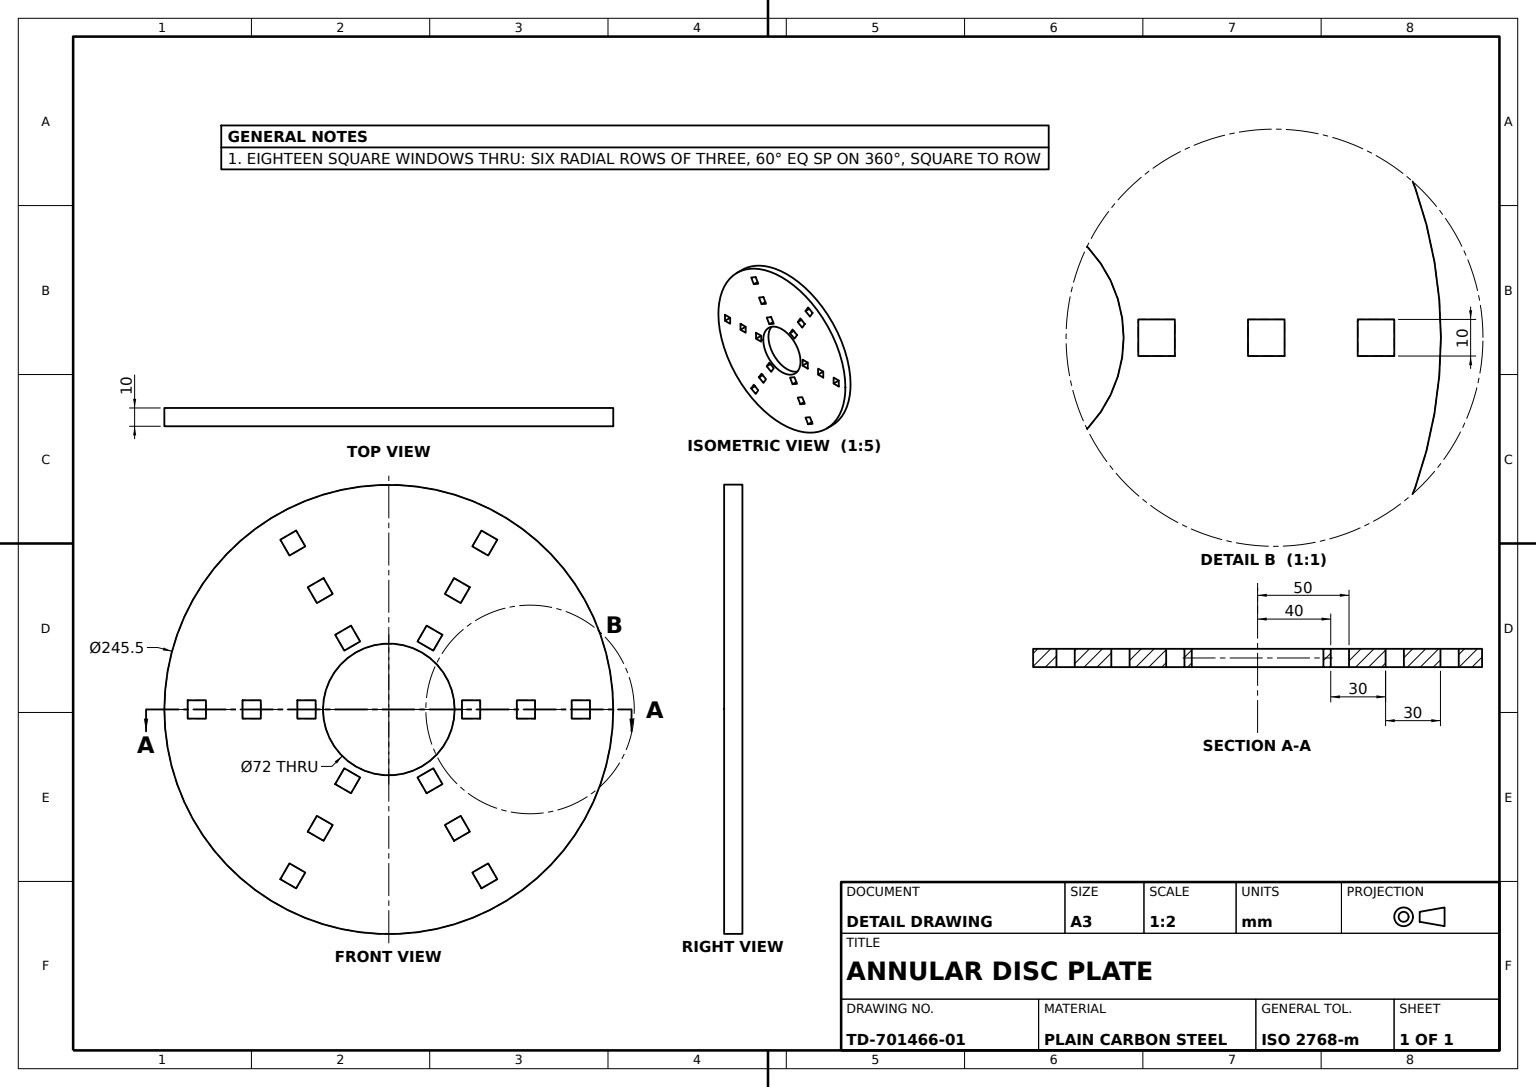
from build123d import *

# Parameters (mm, degrees)
PLATE_PROFILE_245_5_R                        = 122.75
PLATE_DISC_245_5X10_DEPTH                    = 10
CENTRE_BORE_PROFILE_72_R                     = 36
CENTRE_BORE_72_DEPTH                         = 174.882503433
WINDOW_CUT_DEPTH                             = 174.882503433
INNER_WINDOW_CIRCULAR_PATTERN_6X_COUNT       = 6
WINDOW_RADIAL_ROW_3X30_COUNT                 = 3
WINDOW_RADIAL_ROW_3X30_PITCH                 = 30
WINDOW_ROW_CIRCULAR_PATTERN_6X_COPY_1_DEPTH  = 174.882503433
WINDOW_ROW_CIRCULAR_PATTERN_6X_COPY_2_DEPTH  = 174.882503433
WINDOW_ROW_CIRCULAR_PATTERN_6X_COPY_3_DEPTH  = 174.882503433
WINDOW_ROW_CIRCULAR_PATTERN_6X_COPY_4_DEPTH  = 174.882503433
WINDOW_ROW_CIRCULAR_PATTERN_6X_COPY_5_DEPTH  = 174.882503433
WINDOW_ROW_CIRCULAR_PATTERN_6X_COPY_6_DEPTH  = 174.882503433
WINDOW_ROW_CIRCULAR_PATTERN_6X_COPY_7_DEPTH  = 174.882503433
WINDOW_ROW_CIRCULAR_PATTERN_6X_COPY_8_DEPTH  = 174.882503433
WINDOW_ROW_CIRCULAR_PATTERN_6X_COPY_9_DEPTH  = 174.882503433
WINDOW_ROW_CIRCULAR_PATTERN_6X_COPY_10_DEPTH = 174.882503433
WINDOW_ROW_CIRCULAR_PATTERN_6X_COPY_11_DEPTH = 174.882503433
WINDOW_ROW_CIRCULAR_PATTERN_6X_COPY_12_DEPTH = 174.882503433
WINDOW_ROW_CIRCULAR_PATTERN_6X_COPY_13_DEPTH = 174.882503433
WINDOW_ROW_CIRCULAR_PATTERN_6X_COPY_14_DEPTH = 174.882503433
WINDOW_ROW_CIRCULAR_PATTERN_6X_COPY_15_DEPTH = 174.882503433


with BuildPart() as part:
    # Plate Profile Ø245.5 → Plate Disc Ø245.5x10 (new body)
    with BuildSketch(Plane.XY):
        Circle(PLATE_PROFILE_245_5_R)
    extrude(amount=PLATE_DISC_245_5X10_DEPTH)

    # Centre Bore Profile Ø72 → Centre Bore Ø72 (cut, through all)
    with BuildSketch(Plane.XY.offset(10)):
        Circle(CENTRE_BORE_PROFILE_72_R)
    extrude(amount=-CENTRE_BORE_72_DEPTH, mode=Mode.SUBTRACT)

    # Window Profile → Window Cut (cut, through all)
    with BuildSketch(Plane.XY.offset(10)):
        Polygon((50, -5), (50, 5), (40, 5), (40, 0), (40, -5), align=None)
    window_cut = extrude(amount=-WINDOW_CUT_DEPTH, mode=Mode.SUBTRACT)

    # Inner Window Circular Pattern 6x: Window Cut ×6 about axis
    inner_window_circular_pattern_6x_axis = Axis((0, 0, 0), (0, 0, 1))
    for i in range(1, INNER_WINDOW_CIRCULAR_PATTERN_6X_COUNT):
        add(window_cut.rotate(inner_window_circular_pattern_6x_axis, i * 360 / INNER_WINDOW_CIRCULAR_PATTERN_6X_COUNT), mode=Mode.SUBTRACT)

    # Window Radial Row 3x30: Window Cut ×3
    with Locations(*[(i * WINDOW_RADIAL_ROW_3X30_PITCH, 0, 0) for i in range(1, WINDOW_RADIAL_ROW_3X30_COUNT)]):
        add(window_cut, mode=Mode.SUBTRACT)

    # Window Row Circular Pattern 6x copy 1 sk → Window Row Circular Pattern 6x copy 1 (cut, through all)
    with BuildSketch(Plane(origin=(15, 25.980762114, 10), x_dir=(0.5000000000000001, 0.8660254037844386, 0), z_dir=(0, 0, 1))):
        Polygon((50, -5), (50, 5), (40, 5), (40, 0), (40, -5), align=None)
    extrude(amount=-WINDOW_ROW_CIRCULAR_PATTERN_6X_COPY_1_DEPTH, mode=Mode.SUBTRACT)

    # Window Row Circular Pattern 6x copy 2 sk → Window Row Circular Pattern 6x copy 2 (cut, through all)
    with BuildSketch(Plane(origin=(-15, 25.980762114, 10), x_dir=(-0.4999999999999998, 0.8660254037844387, 0), z_dir=(0, 0, 1))):
        Polygon((50, -5), (50, 5), (40, 5), (40, 0), (40, -5), align=None)
    extrude(amount=-WINDOW_ROW_CIRCULAR_PATTERN_6X_COPY_2_DEPTH, mode=Mode.SUBTRACT)

    # Window Row Circular Pattern 6x copy 3 sk → Window Row Circular Pattern 6x copy 3 (cut, through all)
    with BuildSketch(Plane(origin=(-30, 0, 10), x_dir=(-1, 0, 0), z_dir=(0, 0, 1))):
        Polygon((50, -5), (50, 5), (40, 5), (40, 0), (40, -5), align=None)
    extrude(amount=-WINDOW_ROW_CIRCULAR_PATTERN_6X_COPY_3_DEPTH, mode=Mode.SUBTRACT)

    # Window Row Circular Pattern 6x copy 4 sk → Window Row Circular Pattern 6x copy 4 (cut, through all)
    with BuildSketch(Plane(origin=(-15, -25.980762114, 10), x_dir=(-0.5000000000000004, -0.8660254037844384, 0), z_dir=(0, 0, 1))):
        Polygon((50, -5), (50, 5), (40, 5), (40, 0), (40, -5), align=None)
    extrude(amount=-WINDOW_ROW_CIRCULAR_PATTERN_6X_COPY_4_DEPTH, mode=Mode.SUBTRACT)

    # Window Row Circular Pattern 6x copy 5 sk → Window Row Circular Pattern 6x copy 5 (cut, through all)
    with BuildSketch(Plane(origin=(15, -25.980762114, 10), x_dir=(0.5000000000000001, -0.8660254037844386, 0), z_dir=(0, 0, 1))):
        Polygon((50, -5), (50, 5), (40, 5), (40, 0), (40, -5), align=None)
    extrude(amount=-WINDOW_ROW_CIRCULAR_PATTERN_6X_COPY_5_DEPTH, mode=Mode.SUBTRACT)

    # Window Row Circular Pattern 6x copy 6 sk → Window Row Circular Pattern 6x copy 6 (cut, through all)
    with BuildSketch(Plane(origin=(30, 51.961524227, 10), x_dir=(0.5000000000000001, 0.8660254037844386, 0), z_dir=(0, 0, 1))):
        Polygon((50, -5), (50, 5), (40, 5), (40, 0), (40, -5), align=None)
    extrude(amount=-WINDOW_ROW_CIRCULAR_PATTERN_6X_COPY_6_DEPTH, mode=Mode.SUBTRACT)

    # Window Row Circular Pattern 6x copy 7 sk → Window Row Circular Pattern 6x copy 7 (cut, through all)
    with BuildSketch(Plane(origin=(-30, 51.961524227, 10), x_dir=(-0.4999999999999998, 0.8660254037844387, 0), z_dir=(0, 0, 1))):
        Polygon((50, -5), (50, 5), (40, 5), (40, 0), (40, -5), align=None)
    extrude(amount=-WINDOW_ROW_CIRCULAR_PATTERN_6X_COPY_7_DEPTH, mode=Mode.SUBTRACT)

    # Window Row Circular Pattern 6x copy 8 sk → Window Row Circular Pattern 6x copy 8 (cut, through all)
    with BuildSketch(Plane(origin=(-60, 0, 10), x_dir=(-1, 0, 0), z_dir=(0, 0, 1))):
        Polygon((50, -5), (50, 5), (40, 5), (40, 0), (40, -5), align=None)
    extrude(amount=-WINDOW_ROW_CIRCULAR_PATTERN_6X_COPY_8_DEPTH, mode=Mode.SUBTRACT)

    # Window Row Circular Pattern 6x copy 9 sk → Window Row Circular Pattern 6x copy 9 (cut, through all)
    with BuildSketch(Plane(origin=(-30, -51.961524227, 10), x_dir=(-0.5000000000000004, -0.8660254037844384, 0), z_dir=(0, 0, 1))):
        Polygon((50, -5), (50, 5), (40, 5), (40, 0), (40, -5), align=None)
    extrude(amount=-WINDOW_ROW_CIRCULAR_PATTERN_6X_COPY_9_DEPTH, mode=Mode.SUBTRACT)

    # Window Row Circular Pattern 6x copy 10 s → Window Row Circular Pattern 6x copy 10 (cut, through all)
    with BuildSketch(Plane(origin=(30, -51.961524227, 10), x_dir=(0.5000000000000001, -0.8660254037844386, 0), z_dir=(0, 0, 1))):
        Polygon((50, -5), (50, 5), (40, 5), (40, 0), (40, -5), align=None)
    extrude(amount=-WINDOW_ROW_CIRCULAR_PATTERN_6X_COPY_10_DEPTH, mode=Mode.SUBTRACT)

    # Window Row Circular Pattern 6x copy 11 s → Window Row Circular Pattern 6x copy 11 (cut, through all)
    with BuildSketch(Plane(origin=(0, 0, 10), x_dir=(0.5000000000000001, 0.8660254037844386, 0), z_dir=(0, 0, 1))):
        Polygon((50, -5), (50, 5), (40, 5), (40, 0), (40, -5), align=None)
    extrude(amount=-WINDOW_ROW_CIRCULAR_PATTERN_6X_COPY_11_DEPTH, mode=Mode.SUBTRACT)

    # Window Row Circular Pattern 6x copy 12 s → Window Row Circular Pattern 6x copy 12 (cut, through all)
    with BuildSketch(Plane(origin=(0, 0, 10), x_dir=(-0.4999999999999998, 0.8660254037844387, 0), z_dir=(0, 0, 1))):
        Polygon((50, -5), (50, 5), (40, 5), (40, 0), (40, -5), align=None)
    extrude(amount=-WINDOW_ROW_CIRCULAR_PATTERN_6X_COPY_12_DEPTH, mode=Mode.SUBTRACT)

    # Window Row Circular Pattern 6x copy 13 s → Window Row Circular Pattern 6x copy 13 (cut, through all)
    with BuildSketch(Plane(origin=(0, 0, 10), x_dir=(-1, 0, 0), z_dir=(0, 0, 1))):
        Polygon((50, -5), (50, 5), (40, 5), (40, 0), (40, -5), align=None)
    extrude(amount=-WINDOW_ROW_CIRCULAR_PATTERN_6X_COPY_13_DEPTH, mode=Mode.SUBTRACT)

    # Window Row Circular Pattern 6x copy 14 s → Window Row Circular Pattern 6x copy 14 (cut, through all)
    with BuildSketch(Plane(origin=(0, 0, 10), x_dir=(-0.5000000000000004, -0.8660254037844384, 0), z_dir=(0, 0, 1))):
        Polygon((50, -5), (50, 5), (40, 5), (40, 0), (40, -5), align=None)
    extrude(amount=-WINDOW_ROW_CIRCULAR_PATTERN_6X_COPY_14_DEPTH, mode=Mode.SUBTRACT)

    # Window Row Circular Pattern 6x copy 15 s → Window Row Circular Pattern 6x copy 15 (cut, through all)
    with BuildSketch(Plane(origin=(0, 0, 10), x_dir=(0.5000000000000001, -0.8660254037844386, 0), z_dir=(0, 0, 1))):
        Polygon((50, -5), (50, 5), (40, 5), (40, 0), (40, -5), align=None)
    extrude(amount=-WINDOW_ROW_CIRCULAR_PATTERN_6X_COPY_15_DEPTH, mode=Mode.SUBTRACT)


solid = part.part
